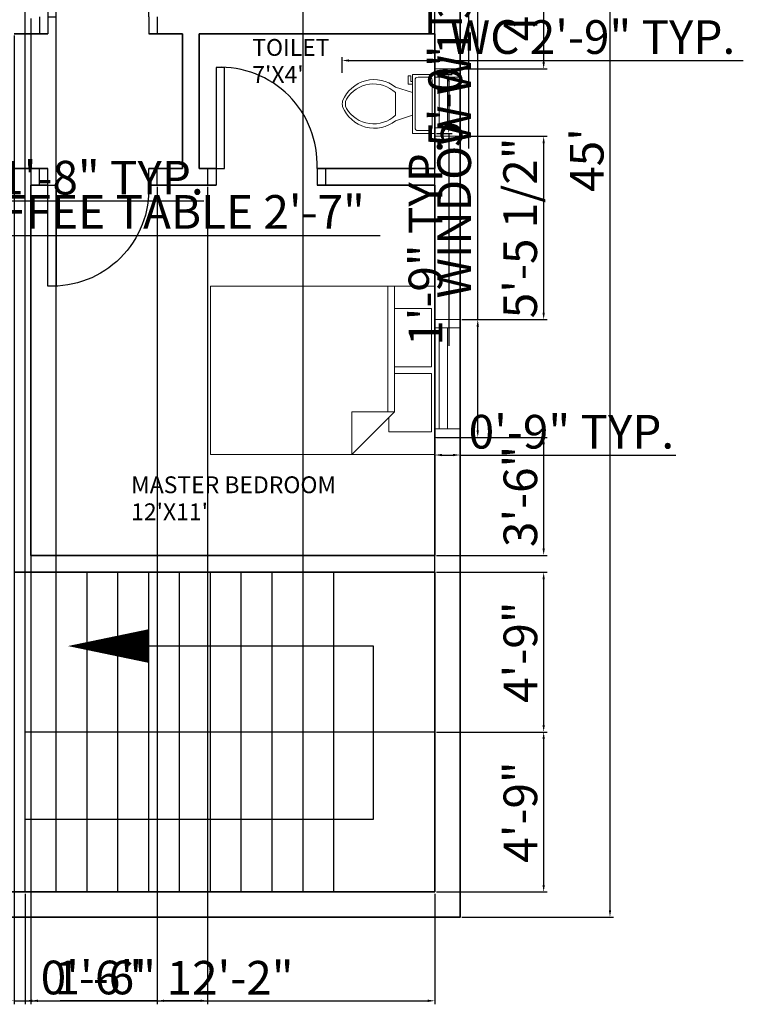
# Model space of a CAD drawing. Units: inches. Extents: x 2011 to 2548, y 530 to 1188.
# Tile 2 of 5: x 2220 to 2478, y 540 to 891. Entities that reach past the tile are written whole.
import ezdxf

# ---------------------------------------------------------------- set-up
doc = ezdxf.new("R2010")
doc.units = ezdxf.units.IN
for name, color, linetype, lineweight in [('A-ANNO-DIMS', 2, 'Continuous', 18), ('A-AREA-IDEN', 7, 'Continuous', 25), ('A-DOOR', 3, 'Continuous', 25), ('A-FLOR-FIXT', 9, 'Continuous', 18), ('A-FLOR-STRS', 7, 'Continuous', 25), ('A-FURN', 8, 'Continuous', 18), ('A-GLAZ', 4, 'Continuous', 18), ('A-WALL', 7, 'Continuous', 35)]:
    doc.layers.add(name, color=color, linetype=linetype, lineweight=lineweight)
doc.styles.get("Standard").update_dxf_attribs({"font": 'arial.ttf'})
doc.dimstyles.new('ISO-25', dxfattribs={"dimtxt": 12, "dimasz": 2.5, "dimexe": 1.25, "dimexo": 0.625, "dimtad": 1, "dimdec": 1, "dimlunit": 3, "dimtxsty": 'Standard', "dimcen": 2.5, "dimadec": 0, "dimazin": 0, "dimtfac": 1, "dimtdec": 1, "dimtmove": 0, "dimatfit": 3, "dimfxl": 1, "dimarcsym": 0})

# ---------------------------------------------------------------- blocks, each defined once
blk = doc.blocks.new('Bed - Queen')
for p, q in [((0, -80.00003), (0, 0)), ((0, 0), (59.99999, 0)), ((59.99999, 0), (59.99999, -80.00003)), ((7.99999, -1.2), (28.79998, -1.2)), ((7.99999, -14.4), (7.99999, -1.2)), ((28.79998, -1.2), (28.79998, -14.4)), ((31.19999, -1.2), (51.99999, -1.2)), ((31.19999, -14.4), (31.19999, -1.2)), ((51.99999, -1.2), (51.99999, -16.4)), ((0, -14.4), (44.8, -14.4)), ((44.8, -16.8), (0, -16.8)), ((59.99999, -29.6), (44.8, -14.4)), ((44.8, -14.4), (44.8, -29.6)), ((51.99999, -16.4), (46.79936, -16.4)), ((44.8, -29.6), (59.99999, -29.6)), ((59.99999, -80.00003), (0, -80.00003))]:
    blk.add_line(p, q)
blk = doc.blocks.new('Toilet - top')
for p, q in [((9.5, -6), (9.5, -2)), ((-10, -8.5), (-8, -8.5)), ((-10, -9.5), (-10, -8.5)), ((-7, -9.5), (-10, -9.5)), ((-8, -8.5), (-8, -8)), ((-7, -8), (-7, -9.5)), ((-4, -8), (-6, -14)), ((4, -8), (6, -14)), ((4, -14), (-4, -14))]:
    blk.add_line(p, q)
blk.add_lwpolyline([(10.5, -8), (10.5, 0), (-10.5, 0), (-10.5, -8)], close=True)
for points in [[(-9.5, -2), (-9.5, -6)], [(8.5, -1), (-8.5, -1)], [(-8.5, -7), (8.5, -7)]]:
    blk.add_lwpolyline(points)
for centre, radius, start, end in [((-8.62, -1.88), 0.884, 81.8699, 188.1301), ((8.62, -1.88), 0.884, 351.8699, 98.1301), ((-8.62, -6.12), 0.884, 171.8699, 278.1301), ((8.62, -6.12), 0.884, 261.8699, 8.1301), ((3.52, -21.58), 12.17, 141.4691, 247.9714), ((4.2, -21.82), 11.33, 136.3677, 238.9468), ((-3.52, -21.58), 12.17, 292.0284, 38.5307), ((-4.2, -21.82), 11.33, 301.053, 43.6321), ((0, -27.88), 4, 245.7318, 294.2682), ((0, -29), 4, 254.8605, 285.1395)]:
    blk.add_arc(centre, radius, start, end)
blk = doc.blocks.new('*D13')
at = {"layer": 'A-ANNO-DIMS', "color": 0, "lineweight": -2, "transparency": 16777216}
for p, q in [((2377.15, 1111.36), (2431.21, 1111.36)), ((2429.96, 1108.86), (2429.96, 573.86)), ((2377.15, 571.36), (2431.21, 571.36))]:
    blk.add_line(p, q, dxfattribs=at)
at = {"layer": 'A-ANNO-DIMS', "color": 0, "transparency": 16777216}
for points in [[(2429.55, 1108.86), (2430.38, 1108.86), (2429.96, 1111.36)], [(2429.55, 573.86), (2430.38, 573.86), (2429.96, 571.36)]]:
    blk.add_solid(points, dxfattribs=at)
at = {"layer": 'Defpoints', "color": 0, "transparency": 16777216}
for p in [(2376.53, 1111.36), (2376.53, 571.36), (2429.96, 571.36)]:
    blk.add_point(p, dxfattribs=at)
at = {"layer": 'A-ANNO-DIMS', "color": 0, "transparency": 16777216, "insert": (2423.24, 841.36), "char_height": 12, "attachment_point": 5, "rotation": 90}
blk.add_mtext("45'", dxfattribs=at)
blk = doc.blocks.new('WIN-36IN')
for p, q in [((0, 42), (9, 42)), ((0, 3), (0, 39)), ((0, 39), (9, 39)), ((1.5, 39), (1.5, 3)), ((4.5, 39), (4.5, 3)), ((9, 39), (9, 3)), ((9, 3), (0, 3)), ((9, 0), (0, 0))]:
    blk.add_line(p, q)
blk = doc.blocks.new('WIN-18IN')
for p, q in [((9, 24), (0, 24)), ((9, 21), (0, 21)), ((0, 21), (0, 3)), ((1.5, 3), (1.5, 21)), ((4.5, 3), (4.5, 21)), ((9, 3), (9, 21)), ((0, 3), (9, 3)), ((0, 0), (9, 0))]:
    blk.add_line(p, q)
blk = doc.blocks.new('DOOR-SWING-36IN-6IN-JAMB')
for p, q in [((0, 6), (0, 0)), ((3, 6), (3, 0)), ((39, 6), (39, 0)), ((42, 6), (42, 0))]:
    blk.add_line(p, q)
blk.add_lwpolyline([(3, 6), (6, 6), (6, 42), (3, 42)], close=True)
blk.add_arc((4.5, 7.5), 34.53, 357.5104, 92.4896)
blk = doc.blocks.new('*D17')
at = {"layer": 'A-ANNO-DIMS', "color": 0, "lineweight": -2, "transparency": 16777216}
for p, q in [((2382.83, 784.45), (2382.83, 969.85)), ((2377.15, 784.45), (2384.08, 784.45)), ((2382.83, 744.95), (2382.83, 781.95)), ((2377.15, 742.45), (2384.08, 742.45))]:
    blk.add_line(p, q, dxfattribs=at)
at = {"layer": 'A-ANNO-DIMS', "color": 0, "transparency": 16777216}
for points in [[(2382.41, 781.95), (2383.24, 781.95), (2382.83, 784.45)], [(2382.41, 744.95), (2383.24, 744.95), (2382.83, 742.45)]]:
    blk.add_solid(points, dxfattribs=at)
at = {"layer": 'Defpoints', "color": 0, "transparency": 16777216}
for p in [(2376.53, 784.45), (2382.83, 784.45), (2376.53, 742.45)]:
    blk.add_point(p, dxfattribs=at)
at = {"layer": 'A-ANNO-DIMS', "color": 0, "transparency": 16777216, "insert": (2375.99, 878.4), "char_height": 12, "attachment_point": 5, "rotation": 90}
blk.add_mtext('WINDOW W1 3\'-6" TYP.', dxfattribs=at)
blk = doc.blocks.new('*D18')
at = {"layer": 'A-ANNO-DIMS', "color": 0, "lineweight": -2, "transparency": 16777216}
for p, q in [((2367.53, 741.82), (2367.53, 734.9)), ((2376.53, 741.82), (2376.53, 734.9)), ((2370.03, 736.15), (2374.03, 736.15)), ((2376.53, 736.15), (2453.42, 736.15))]:
    blk.add_line(p, q, dxfattribs=at)
at = {"layer": 'A-ANNO-DIMS', "color": 0, "transparency": 16777216}
for points in [[(2370.03, 736.56), (2370.03, 735.73), (2367.53, 736.15)], [(2374.03, 736.56), (2374.03, 735.73), (2376.53, 736.15)]]:
    blk.add_solid(points, dxfattribs=at)
at = {"layer": 'Defpoints', "color": 0, "transparency": 16777216}
for p in [(2367.53, 742.45), (2376.53, 742.45), (2376.53, 736.15)]:
    blk.add_point(p, dxfattribs=at)
at = {"layer": 'A-ANNO-DIMS', "color": 0, "transparency": 16777216, "insert": (2416.22, 742.9), "char_height": 12, "attachment_point": 5}
blk.add_mtext('0\'-9" TYP.', dxfattribs=at)
blk = doc.blocks.new('*D23')
at = {"layer": 'A-ANNO-DIMS', "color": 0, "lineweight": -2, "transparency": 16777216}
for p, q in [((2334.48, 872.46), (2334.48, 878.04)), ((2367.53, 872.46), (2367.53, 878.04)), ((2336.98, 876.79), (2365.03, 876.79)), ((2367.53, 876.79), (2477.5, 876.79))]:
    blk.add_line(p, q, dxfattribs=at)
at = {"layer": 'A-ANNO-DIMS', "color": 0, "transparency": 16777216}
for points in [[(2336.98, 877.21), (2336.98, 876.38), (2334.48, 876.79)], [(2365.03, 877.21), (2365.03, 876.38), (2367.53, 876.79)]]:
    blk.add_solid(points, dxfattribs=at)
at = {"layer": 'Defpoints', "color": 0, "transparency": 16777216}
for p in [(2367.53, 876.79), (2334.48, 871.84), (2367.53, 871.84)]:
    blk.add_point(p, dxfattribs=at)
at = {"layer": 'A-ANNO-DIMS', "color": 0, "transparency": 16777216, "insert": (2423.76, 883.62), "char_height": 12, "attachment_point": 5}
blk.add_mtext('WC 2\'-9" TYP.', dxfattribs=at)
blk = doc.blocks.new('*D24')
at = {"layer": 'A-ANNO-DIMS', "color": 0, "lineweight": -2, "transparency": 16777216}
for p, q in [((2368.15, 871.84), (2373.73, 871.84)), ((2372.48, 869.34), (2372.48, 853.34)), ((2368.15, 850.84), (2373.73, 850.84)), ((2372.48, 850.84), (2372.48, 775.07))]:
    blk.add_line(p, q, dxfattribs=at)
at = {"layer": 'A-ANNO-DIMS', "color": 0, "transparency": 16777216}
for points in [[(2372.07, 869.34), (2372.9, 869.34), (2372.48, 871.84)], [(2372.07, 853.34), (2372.9, 853.34), (2372.48, 850.84)]]:
    blk.add_solid(points, dxfattribs=at)
at = {"layer": 'Defpoints', "color": 0, "transparency": 16777216}
for p in [(2367.53, 871.84), (2367.53, 850.84), (2372.48, 850.84)]:
    blk.add_point(p, dxfattribs=at)
at = {"layer": 'A-ANNO-DIMS', "color": 0, "transparency": 16777216, "insert": (2365.73, 811.7), "char_height": 12, "attachment_point": 5, "rotation": 90}
blk.add_mtext('1\'-9" TYP.', dxfattribs=at)
blk = doc.blocks.new('*D26')
at = {"layer": 'A-ANNO-DIMS', "color": 0, "lineweight": -2, "transparency": 16777216}
for p, q in [((2368.15, 982.36), (2380.78, 982.36)), ((2379.53, 979.86), (2379.53, 924.86)), ((2368.15, 922.36), (2380.78, 922.36)), ((2379.53, 922.36), (2379.53, 845.46))]:
    blk.add_line(p, q, dxfattribs=at)
at = {"layer": 'A-ANNO-DIMS', "color": 0, "transparency": 16777216}
for points in [[(2379.11, 979.86), (2379.94, 979.86), (2379.53, 982.36)], [(2379.11, 924.86), (2379.94, 924.86), (2379.53, 922.36)]]:
    blk.add_solid(points, dxfattribs=at)
at = {"layer": 'Defpoints', "color": 0, "transparency": 16777216}
for p in [(2367.53, 982.36), (2367.53, 922.36), (2379.53, 922.36)]:
    blk.add_point(p, dxfattribs=at)
at = {"layer": 'A-ANNO-DIMS', "color": 0, "transparency": 16777216, "insert": (2372.78, 882.66), "char_height": 12, "attachment_point": 5, "rotation": 90}
blk.add_mtext('5\'-0" TYP.', dxfattribs=at)
blk = doc.blocks.new('*D27')
at = {"layer": 'A-ANNO-DIMS', "color": 0, "lineweight": -2, "transparency": 16777216}
for p, q in [((2210, 821.8), (2215.55, 821.8)), ((2214.3, 819.3), (2214.3, 791.47)), ((2210, 788.97), (2215.55, 788.97)), ((2214.3, 788.97), (2214.3, 619.44))]:
    blk.add_line(p, q, dxfattribs=at)
at = {"layer": 'A-ANNO-DIMS', "color": 0, "transparency": 16777216}
for points in [[(2213.88, 819.3), (2214.72, 819.3), (2214.3, 821.8)], [(2213.88, 791.47), (2214.72, 791.47), (2214.3, 788.97)]]:
    blk.add_solid(points, dxfattribs=at)
at = {"layer": 'Defpoints', "color": 0, "transparency": 16777216}
for p in [(2209.38, 821.8), (2209.38, 788.97), (2214.3, 788.97)]:
    blk.add_point(p, dxfattribs=at)
at = {"layer": 'A-ANNO-DIMS', "color": 0, "transparency": 16777216, "insert": (2207.47, 702.96), "char_height": 12, "attachment_point": 5, "rotation": 90}
blk.add_mtext('LOVESEAT 2\'-9" TYP.', dxfattribs=at)
blk = doc.blocks.new('*D28')
at = {"layer": 'A-ANNO-DIMS', "color": 0, "lineweight": -2, "transparency": 16777216}
for p, q in [((2189.31, 822.43), (2189.31, 827.98)), ((2191.81, 826.73), (2206.88, 826.73)), ((2209.38, 822.43), (2209.38, 827.98)), ((2209.38, 826.73), (2285.14, 826.73))]:
    blk.add_line(p, q, dxfattribs=at)
at = {"layer": 'A-ANNO-DIMS', "color": 0, "transparency": 16777216}
for points in [[(2191.81, 827.15), (2191.81, 826.31), (2189.31, 826.73)], [(2206.88, 827.15), (2206.88, 826.31), (2209.38, 826.73)]]:
    blk.add_solid(points, dxfattribs=at)
at = {"layer": 'Defpoints', "color": 0, "transparency": 16777216}
for p in [(2209.38, 826.73), (2189.31, 821.8), (2209.38, 821.8)]:
    blk.add_point(p, dxfattribs=at)
at = {"layer": 'A-ANNO-DIMS', "color": 0, "transparency": 16777216, "insert": (2248.51, 833.48), "char_height": 12, "attachment_point": 5}
blk.add_mtext('1\'-8" TYP.', dxfattribs=at)
blk = doc.blocks.new('*D39')
at = {"layer": 'A-ANNO-DIMS', "color": 0, "lineweight": -2, "transparency": 16777216}
for p, q in [((2150.94, 810.39), (2150.94, 815.69)), ((2153.44, 814.44), (2179.61, 814.44)), ((2182.11, 810.39), (2182.11, 815.69)), ((2182.11, 814.44), (2348.03, 814.44))]:
    blk.add_line(p, q, dxfattribs=at)
at = {"layer": 'A-ANNO-DIMS', "color": 0, "transparency": 16777216}
for points in [[(2153.44, 814.85), (2153.44, 814.02), (2150.94, 814.44)], [(2179.61, 814.85), (2179.61, 814.02), (2182.11, 814.44)]]:
    blk.add_solid(points, dxfattribs=at)
at = {"layer": 'Defpoints', "color": 0, "transparency": 16777216}
for p in [(2182.11, 814.44), (2150.94, 809.76), (2182.11, 809.76)]:
    blk.add_point(p, dxfattribs=at)
at = {"layer": 'A-ANNO-DIMS', "color": 0, "transparency": 16777216, "insert": (2266.32, 821.27), "char_height": 12, "attachment_point": 5}
blk.add_mtext('COFFEE TABLE 2\'-7"', dxfattribs=at)
blk = doc.blocks.new('*D43')
at = {"layer": 'A-ANNO-DIMS', "color": 0, "lineweight": -2, "transparency": 16777216}
for p, q in [((2221.53, 579.73), (2221.53, 540.31)), ((2367.53, 579.73), (2367.53, 540.31)), ((2224.03, 541.56), (2365.03, 541.56))]:
    blk.add_line(p, q, dxfattribs=at)
at = {"layer": 'A-ANNO-DIMS', "color": 0, "transparency": 16777216}
for points in [[(2224.03, 541.98), (2224.03, 541.14), (2221.53, 541.56)], [(2365.03, 541.98), (2365.03, 541.14), (2367.53, 541.56)]]:
    blk.add_solid(points, dxfattribs=at)
at = {"layer": 'Defpoints', "color": 0, "transparency": 16777216}
for p in [(2221.53, 580.36), (2367.53, 580.36), (2367.53, 541.56)]:
    blk.add_point(p, dxfattribs=at)
at = {"layer": 'A-ANNO-DIMS', "color": 0, "transparency": 16777216, "insert": (2294.53, 548.21), "char_height": 12, "attachment_point": 5}
blk.add_mtext('12\'-2"', dxfattribs=at)
blk = doc.blocks.new('*D44')
at = {"layer": 'A-ANNO-DIMS', "color": 0, "lineweight": -2, "transparency": 16777216}
for p, q in [((2368.15, 637.36), (2407.58, 637.36)), ((2406.33, 582.86), (2406.33, 634.86)), ((2368.15, 580.36), (2407.58, 580.36))]:
    blk.add_line(p, q, dxfattribs=at)
at = {"layer": 'A-ANNO-DIMS', "color": 0, "transparency": 16777216}
for points in [[(2405.91, 634.86), (2406.74, 634.86), (2406.33, 637.36)], [(2405.91, 582.86), (2406.74, 582.86), (2406.33, 580.36)]]:
    blk.add_solid(points, dxfattribs=at)
at = {"layer": 'Defpoints', "color": 0, "transparency": 16777216}
for p in [(2367.53, 637.36), (2406.33, 637.36), (2367.53, 580.36)]:
    blk.add_point(p, dxfattribs=at)
at = {"layer": 'A-ANNO-DIMS', "color": 0, "transparency": 16777216, "insert": (2399.58, 608.86), "char_height": 12, "attachment_point": 5, "rotation": 90}
blk.add_mtext('4\'-9"', dxfattribs=at)
blk = doc.blocks.new('*D46')
at = {"layer": 'A-ANNO-DIMS', "color": 0, "lineweight": -2, "transparency": 16777216}
for p, q in [((2221.53, 580.98), (2221.53, 1142.41)), ((2224.03, 1141.16), (2230.03, 1141.16)), ((2232.53, 580.98), (2232.53, 1142.41)), ((2232.53, 1141.16), (2277.5, 1141.16))]:
    blk.add_line(p, q, dxfattribs=at)
at = {"layer": 'A-ANNO-DIMS', "color": 0, "transparency": 16777216}
for points in [[(2224.03, 1141.58), (2224.03, 1140.74), (2221.53, 1141.16)], [(2230.03, 1141.58), (2230.03, 1140.74), (2232.53, 1141.16)]]:
    blk.add_solid(points, dxfattribs=at)
at = {"layer": 'Defpoints', "color": 0, "transparency": 16777216}
for p in [(2232.53, 1141.16), (2221.53, 580.36), (2232.53, 580.36)]:
    blk.add_point(p, dxfattribs=at)
at = {"layer": 'A-ANNO-DIMS', "color": 0, "transparency": 16777216, "insert": (2256.26, 1147.91), "char_height": 12, "attachment_point": 5}
blk.add_mtext('0\'-11"', dxfattribs=at)
blk = doc.blocks.new('*D50')
at = {"layer": 'A-ANNO-DIMS', "color": 0, "lineweight": -2, "transparency": 16777216}
for p, q in [((2368.15, 742.45), (2407.58, 742.45)), ((2406.33, 702.86), (2406.33, 739.95)), ((2368.15, 700.36), (2407.58, 700.36))]:
    blk.add_line(p, q, dxfattribs=at)
at = {"layer": 'A-ANNO-DIMS', "color": 0, "transparency": 16777216}
for points in [[(2405.91, 739.95), (2406.74, 739.95), (2406.33, 742.45)], [(2405.91, 702.86), (2406.74, 702.86), (2406.33, 700.36)]]:
    blk.add_solid(points, dxfattribs=at)
at = {"layer": 'Defpoints', "color": 0, "transparency": 16777216}
for p in [(2367.53, 742.45), (2406.33, 742.45), (2367.53, 700.36)]:
    blk.add_point(p, dxfattribs=at)
at = {"layer": 'A-ANNO-DIMS', "color": 0, "transparency": 16777216, "insert": (2399.57, 721.4), "char_height": 12, "attachment_point": 5, "rotation": 90}
blk.add_mtext('3\'-6"', dxfattribs=at)
blk = doc.blocks.new('*D51')
at = {"layer": 'A-ANNO-DIMS', "color": 0, "lineweight": -2, "transparency": 16777216}
for p, q in [((2377.15, 849.81), (2407.58, 849.81)), ((2406.33, 786.95), (2406.33, 847.31)), ((2377.15, 784.45), (2407.58, 784.45))]:
    blk.add_line(p, q, dxfattribs=at)
at = {"layer": 'A-ANNO-DIMS', "color": 0, "transparency": 16777216}
for points in [[(2405.91, 847.31), (2406.74, 847.31), (2406.33, 849.81)], [(2405.91, 786.95), (2406.74, 786.95), (2406.33, 784.45)]]:
    blk.add_solid(points, dxfattribs=at)
at = {"layer": 'Defpoints', "color": 0, "transparency": 16777216}
for p in [(2376.53, 849.81), (2406.33, 849.81), (2376.53, 784.45)]:
    blk.add_point(p, dxfattribs=at)
at = {"layer": 'A-ANNO-DIMS', "color": 0, "transparency": 16777216, "insert": (2399.5, 817.13), "char_height": 12, "attachment_point": 5, "rotation": 90}
blk.add_mtext('5\'-5 1/2"', dxfattribs=at)
blk = doc.blocks.new('*D52')
at = {"layer": 'A-ANNO-DIMS', "color": 0, "lineweight": -2, "transparency": 16777216}
for p, q in [((2377.15, 929.66), (2407.58, 929.66)), ((2406.33, 876.31), (2406.33, 927.16)), ((2377.15, 873.81), (2407.58, 873.81))]:
    blk.add_line(p, q, dxfattribs=at)
at = {"layer": 'A-ANNO-DIMS', "color": 0, "transparency": 16777216}
for points in [[(2405.91, 927.16), (2406.74, 927.16), (2406.33, 929.66)], [(2405.91, 876.31), (2406.74, 876.31), (2406.33, 873.81)]]:
    blk.add_solid(points, dxfattribs=at)
at = {"layer": 'Defpoints', "color": 0, "transparency": 16777216}
for p in [(2376.53, 929.66), (2406.33, 929.66), (2376.53, 873.81)]:
    blk.add_point(p, dxfattribs=at)
at = {"layer": 'A-ANNO-DIMS', "color": 0, "transparency": 16777216, "insert": (2399.58, 901.74), "char_height": 12, "attachment_point": 5, "rotation": 90}
blk.add_mtext('4\'-8"', dxfattribs=at)
blk = doc.blocks.new('*D54')
at = {"layer": 'A-ANNO-DIMS', "color": 0, "lineweight": -2, "transparency": 16777216}
for p, q in [((2223.53, 891.73), (2223.53, 540.31)), ((2217.53, 885.73), (2217.53, 540.31)), ((2215.03, 541.56), (2212.53, 541.56)), ((2217.53, 541.56), (2223.53, 541.56)), ((2226.03, 541.56), (2261.68, 541.56))]:
    blk.add_line(p, q, dxfattribs=at)
at = {"layer": 'A-ANNO-DIMS', "color": 0, "transparency": 16777216}
for points in [[(2215.03, 541.98), (2215.03, 541.14), (2217.53, 541.56)], [(2226.03, 541.98), (2226.03, 541.14), (2223.53, 541.56)]]:
    blk.add_solid(points, dxfattribs=at)
at = {"layer": 'Defpoints', "color": 0, "transparency": 16777216}
for p in [(2223.53, 892.36), (2217.53, 886.36), (2223.53, 541.56)]:
    blk.add_point(p, dxfattribs=at)
at = {"layer": 'A-ANNO-DIMS', "color": 0, "transparency": 16777216, "insert": (2245.1, 548.31), "char_height": 12, "attachment_point": 5}
blk.add_mtext('0\'-6"', dxfattribs=at)
blk = doc.blocks.new('*D60')
at = {"layer": 'A-ANNO-DIMS', "color": 0, "lineweight": -2, "transparency": 16777216}
for p, q in [((2320.53, 580.98), (2320.53, 1142.41)), ((2323.03, 1141.16), (2365.03, 1141.16)), ((2367.53, 580.98), (2367.53, 1142.41))]:
    blk.add_line(p, q, dxfattribs=at)
at = {"layer": 'A-ANNO-DIMS', "color": 0, "transparency": 16777216}
for points in [[(2323.03, 1141.58), (2323.03, 1140.74), (2320.53, 1141.16)], [(2365.03, 1141.58), (2365.03, 1140.74), (2367.53, 1141.16)]]:
    blk.add_solid(points, dxfattribs=at)
at = {"layer": 'Defpoints', "color": 0, "transparency": 16777216}
for p in [(2367.53, 1141.16), (2320.53, 580.36), (2367.53, 580.36)]:
    blk.add_point(p, dxfattribs=at)
at = {"layer": 'A-ANNO-DIMS', "color": 0, "transparency": 16777216, "insert": (2344.03, 1147.91), "char_height": 12, "attachment_point": 5}
blk.add_mtext('3\'-11"', dxfattribs=at)
blk = doc.blocks.new('*D61')
at = {"layer": 'A-ANNO-DIMS', "color": 0, "lineweight": -2, "transparency": 16777216}
for p, q in [((2368.15, 694.36), (2407.58, 694.36)), ((2406.33, 639.86), (2406.33, 691.86)), ((2368.15, 637.36), (2407.58, 637.36))]:
    blk.add_line(p, q, dxfattribs=at)
at = {"layer": 'A-ANNO-DIMS', "color": 0, "transparency": 16777216}
for points in [[(2405.91, 691.86), (2406.74, 691.86), (2406.33, 694.36)], [(2405.91, 639.86), (2406.74, 639.86), (2406.33, 637.36)]]:
    blk.add_solid(points, dxfattribs=at)
at = {"layer": 'Defpoints', "color": 0, "transparency": 16777216}
for p in [(2367.53, 694.36), (2406.33, 694.36), (2367.53, 637.36)]:
    blk.add_point(p, dxfattribs=at)
at = {"layer": 'A-ANNO-DIMS', "color": 0, "transparency": 16777216, "insert": (2399.58, 665.86), "char_height": 12, "attachment_point": 5, "rotation": 90}
blk.add_mtext('4\'-9"', dxfattribs=at)
blk = doc.blocks.new('*D63')
at = {"layer": 'A-ANNO-DIMS', "color": 0, "lineweight": -2, "transparency": 16777216}
for p, q in [((2268.53, 831.73), (2268.53, 540.31)), ((2286.53, 831.73), (2286.53, 540.31)), ((2268.53, 541.56), (2234.01, 541.56)), ((2284.03, 541.56), (2271.03, 541.56))]:
    blk.add_line(p, q, dxfattribs=at)
at = {"layer": 'A-ANNO-DIMS', "color": 0, "transparency": 16777216}
for points in [[(2271.03, 541.98), (2271.03, 541.14), (2268.53, 541.56)], [(2284.03, 541.98), (2284.03, 541.14), (2286.53, 541.56)]]:
    blk.add_solid(points, dxfattribs=at)
at = {"layer": 'Defpoints', "color": 0, "transparency": 16777216}
for p in [(2268.53, 832.36), (2286.53, 832.36), (2268.53, 541.56)]:
    blk.add_point(p, dxfattribs=at)
at = {"layer": 'A-ANNO-DIMS', "color": 0, "transparency": 16777216, "insert": (2250.02, 548.31), "char_height": 12, "attachment_point": 5}
blk.add_mtext('1\'-6"', dxfattribs=at)

msp = doc.modelspace()

# ---------------------------------------------------------------- linework, layer by layer
at = {"layer": 'A-FLOR-STRS'}
for p, q in [((2221.53, 580.36), (2221.53, 694.36)), ((2232.53, 580.36), (2232.53, 694.36)), ((2243.53, 580.36), (2243.53, 694.36)), ((2254.53, 580.36), (2254.53, 694.36)), ((2265.53, 580.36), (2265.53, 694.36)), ((2276.53, 580.36), (2276.53, 694.36)), ((2287.53, 580.36), (2287.53, 694.36)), ((2298.53, 580.36), (2298.53, 694.36)), ((2309.53, 580.36), (2309.53, 694.36)), ((2320.53, 580.36), (2320.53, 694.36)), ((2331.53, 580.36), (2331.53, 694.36)), ((2367.53, 637.36), (2221.53, 637.36))]:
    msp.add_line(p, q, dxfattribs=at)
msp.add_lwpolyline([(2265.53, 668.04, 12, 0, 0), (2236.71, 668.04, 0, 0, 0)], format="xyseb", dxfattribs=at)
msp.add_lwpolyline([(2221.53, 606.3), (2345.63, 606.3), (2345.63, 668.04), (2265.53, 668.04)], dxfattribs=at)
at = {"layer": 'A-WALL'}
for p, q in [((2229.53, 886.36), (2217.53, 886.36)), ((2277.53, 886.36), (2265.53, 886.36)), ((2277.53, 838.36), (2277.53, 886.36)), ((2367.53, 886.36), (2283.53, 886.36)), ((2283.53, 838.36), (2283.53, 886.36)), ((2367.53, 838.36), (2367.53, 886.36)), ((2229.53, 838.36), (2217.53, 838.36)), ((2277.53, 838.36), (2265.53, 838.36)), ((2289.53, 838.36), (2283.53, 838.36)), ((2367.53, 838.36), (2325.53, 838.36)), ((2223.53, 700.36), (2223.53, 832.36)), ((2229.53, 832.36), (2223.53, 832.36)), ((2289.53, 832.36), (2265.53, 832.36)), ((2367.53, 832.36), (2325.53, 832.36)), ((2367.53, 700.36), (2367.53, 832.36)), ((2367.53, 700.36), (2223.53, 700.36)), ((2367.53, 694.36), (2217.53, 694.36)), ((2367.53, 580.36), (2367.53, 694.36)), ((2085.53, 580.36), (2367.53, 580.36))]:
    msp.add_line(p, q, dxfattribs=at)
msp.add_lwpolyline([(2076.53, 1060.36), (2076.53, 571.36), (2376.53, 571.36), (2376.53, 1111.36), (2076.53, 1111.36), (2076.53, 1096.36)], dxfattribs=at)

# ---------------------------------------------------------------- block references
at = {"layer": 'A-DOOR'}
for p in [(2226.53, 886.36), (2286.53, 832.36)]:
    msp.add_blockref('DOOR-SWING-36IN-6IN-JAMB', p, dxfattribs=at)
at = {"layer": 'A-DOOR', "extrusion": (0, 0, -1), "zscale": -1, "rotation": 180}
msp.add_blockref('DOOR-SWING-36IN-6IN-JAMB', (-2226.53, 838.36), dxfattribs=at)
at = {"layer": 'A-FLOR-FIXT', "rotation": 270}
msp.add_blockref('Toilet - top', (2367.53, 861.34), dxfattribs=at)
at = {"layer": 'A-FURN', "rotation": 270}
msp.add_blockref('Bed - Queen', (2367.53, 796.36), dxfattribs=at)
at = {"layer": 'A-GLAZ'}
for name, p in [('WIN-18IN', (2367.53, 849.81)), ('WIN-36IN', (2367.53, 742.45))]:
    msp.add_blockref(name, p, dxfattribs=at)

# ---------------------------------------------------------------- texts
at = {"layer": 'A-AREA-IDEN'}
for s, p in [('TOILET', (2302.43, 878.47)), ("7'X4'", (2302.43, 868.83)), ('MASTER BEDROOM', (2259.25, 722.54)), ("12'X11'", (2259.25, 712.9))]:
    msp.add_text(s, height=6, dxfattribs=at).set_placement(p)

# ---------------------------------------------------------------- dimensions: what is measured, and where the dimension line sits
at = {"layer": 'A-ANNO-DIMS'}
for base, p1, p2, picture, middle in [((2232.53, 1141.16), (2221.53, 580.36), (2232.53, 580.36), '*D46', (2256.26, 1147.91)), ((2367.53, 1141.16), (2320.53, 580.36), (2367.53, 580.36), '*D60', (2344.03, 1147.91)), ((2223.53, 541.56), (2217.53, 886.36), (2223.53, 892.36), '*D54', (2245.1, 548.31)), ((2268.53, 541.56), (2286.53, 832.36), (2268.53, 832.36), '*D63', (2250.02, 548.31)), ((2367.53, 541.56), (2221.53, 580.36), (2367.53, 580.36), '*D43', (2294.53, 548.21))]:
    dim = msp.add_linear_dim(base=base, p1=p1, p2=p2, dimstyle='ISO-25', override={"dimdec": 1, "dimlfac": 1, "dimrnd": 0, "dimzin": 1, "dimdsep": 46, "dimlunit": 4, "dimfrac": 2}, dxfattribs=at)
    dim.commit()
    dim.dimension.update_dxf_attribs({"geometry": picture, "text_midpoint": middle})
for base, p1, p2, override, picture, middle in [((2429.96, 571.36), (2376.53, 1111.36), (2376.53, 571.36), {"dimclrd": 0, "dimclre": 0, "dimclrt": 0}, '*D13', (2423.24, 841.36)), ((2406.327, 929.6645), (2376.527, 873.8101), (2376.527, 929.6645), {"dimdec": 1, "dimlfac": 1, "dimrnd": 0, "dimzin": 1, "dimdsep": 46, "dimlunit": 4, "dimfrac": 2}, '*D52', (2399.5751, 901.7373)), ((2406.33, 849.81), (2376.53, 784.45), (2376.53, 849.81), {"dimdec": 1, "dimlfac": 1, "dimrnd": 0, "dimzin": 1, "dimdsep": 46, "dimlunit": 4, "dimfrac": 2}, '*D51', (2399.5, 817.13)), ((2406.33, 742.45), (2367.53, 700.36), (2367.53, 742.45), {"dimdec": 1, "dimlfac": 1, "dimrnd": 0, "dimzin": 1, "dimdsep": 46, "dimlunit": 4, "dimfrac": 2}, '*D50', (2399.57, 721.4)), ((2406.33, 694.36), (2367.53, 637.36), (2367.53, 694.36), {"dimdec": 1, "dimlfac": 1, "dimrnd": 0, "dimzin": 1, "dimdsep": 46, "dimlunit": 4, "dimfrac": 2}, '*D61', (2399.58, 665.86)), ((2406.33, 637.36), (2367.53, 580.36), (2367.53, 637.36), {"dimdec": 1, "dimlfac": 1, "dimrnd": 0, "dimzin": 1, "dimdsep": 46, "dimlunit": 4, "dimfrac": 2}, '*D44', (2399.58, 608.86))]:
    dim = msp.add_linear_dim(base=base, p1=p1, p2=p2, angle=90, dimstyle='ISO-25', override=override, dxfattribs=at)
    dim.commit()
    dim.dimension.update_dxf_attribs({"geometry": picture, "text_midpoint": middle})
for base, p1, p2, angle, text, picture, middle in [((2379.53, 922.36), (2367.53, 982.36), (2367.53, 922.36), 270, '<> TYP.', '*D26', (2372.78, 882.66)), ((2382.83, 784.45), (2376.53, 742.45), (2376.53, 784.45), 90, 'WINDOW W1 <> TYP.', '*D17', (2375.99, 878.4)), ((2372.48, 850.84), (2367.53, 871.84), (2367.53, 850.84), 270, '<> TYP.', '*D24', (2365.73, 811.7)), ((2214.3, 788.97), (2209.38, 821.8), (2209.38, 788.97), 270, 'LOVESEAT <> TYP.', '*D27', (2207.47, 702.96))]:
    dim = msp.add_linear_dim(base=base, p1=p1, p2=p2, angle=angle, text=text, dimstyle='ISO-25', override={"dimdec": 1, "dimlfac": 1, "dimrnd": 0, "dimzin": 1, "dimdsep": 46, "dimlunit": 4, "dimfrac": 2}, dxfattribs=at)
    dim.commit()
    dim.dimension.update_dxf_attribs({"geometry": picture, "text_midpoint": middle})
for base, p1, p2, text, picture, middle in [((2367.527, 876.7924), (2334.4807, 871.8355), (2367.527, 871.8355), 'WC <> TYP.', '*D23', (2423.7639, 883.622)), ((2209.38, 826.73), (2189.31, 821.8), (2209.38, 821.8), '<> TYP.', '*D28', (2248.51, 833.48)), ((2182.11, 814.44), (2150.94, 809.76), (2182.11, 809.76), 'COFFEE TABLE <>', '*D39', (2266.32, 821.27)), ((2376.53, 736.15), (2367.53, 742.45), (2376.53, 742.45), '<> TYP.', '*D18', (2416.22, 742.9))]:
    dim = msp.add_linear_dim(base=base, p1=p1, p2=p2, text=text, dimstyle='ISO-25', override={"dimdec": 1, "dimlfac": 1, "dimrnd": 0, "dimzin": 1, "dimdsep": 46, "dimlunit": 4, "dimfrac": 2}, dxfattribs=at)
    dim.commit()
    dim.dimension.update_dxf_attribs({"geometry": picture, "text_midpoint": middle})

doc.saveas('drawing.dxf')
